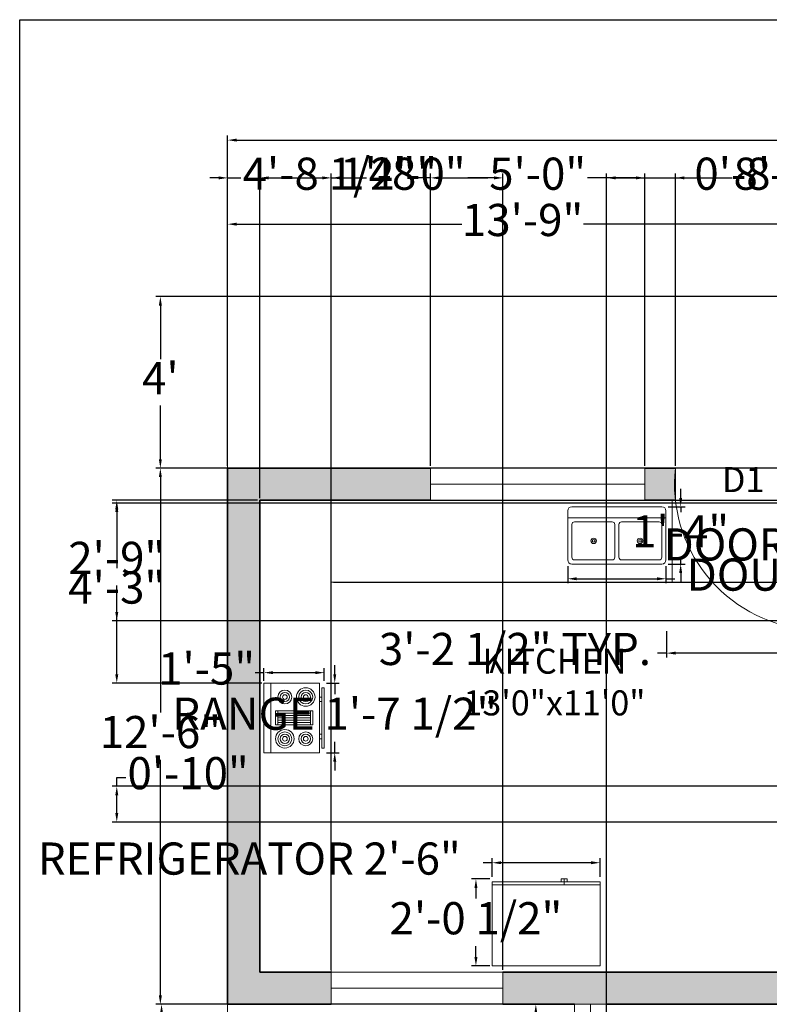
# Model space of a CAD drawing. Units: inches. Extents: x 1942 to 2601, y 2026 to 2623.
# Tile 2 of 5: x 1942 to 2151, y 2348 to 2623. Entities that reach past the tile are written whole.
import ezdxf

# ---------------------------------------------------------------- set-up
doc = ezdxf.new("R2010")
doc.units = ezdxf.units.IN
doc.linetypes.add('ACAD_ISO02W100', pattern=[15, 12, -3])
for name, color, linetype, lineweight in [('A-ANNO-DIMS', 2, 'Continuous', 18), ('A-ANNO-TEXT', 7, 'Continuous', 18), ('A-ANNO-TTLB', 7, 'Continuous', 25), ('A-AREA-IDEN', 7, 'Continuous', 25), ('A-DOOR', 4, 'Continuous', 18), ('A-EQPM', 8, 'Continuous', 18), ('A-FLOR-CASE', 8, 'Continuous', 18), ('A-FLOR-FIXT', 8, 'Continuous', 18), ('A-FLOR-OTLN', 8, 'ACAD_ISO02W100', 13), ('A-GLAZ', 2, 'Continuous', 18), ('A-WALL', 7, 'Continuous', 35), ('A-WALL-PATT', 7, 'Continuous', 13)]:
    doc.layers.add(name, color=color, linetype=linetype, lineweight=lineweight)
doc.styles.get("Standard").update_dxf_attribs({"font": 'arial.ttf'})
doc.dimstyles.new('ISO-25', dxfattribs={"dimtxt": 9, "dimasz": 2.5, "dimexe": 1.25, "dimexo": 0.625, "dimgap": 2, "dimtad": 0, "dimtih": 1, "dimtoh": 1, "dimdec": 1, "dimlunit": 4, "dimtxsty": 'Standard', "dimcen": 2.5, "dimadec": 0, "dimazin": 0, "dimtfac": 0.5, "dimtdec": 1, "dimtmove": 0, "dimatfit": 3, "dimfxl": 1, "dimarcsym": 0})

# ---------------------------------------------------------------- blocks, each defined once
blk = doc.blocks.new('Sink-double - 36 in top')
for p, q in [((-18, -4), (18, -4)), ((-0.75, -18.5), (-0.75, -6.5)), ((0.75, -6.5), (0.75, -18.5))]:
    blk.add_line(p, q)
for points in [[(-16.5, 0), (16.5, 0)], [(-18, -19.5), (-18, -1.5)], [(18, -1.5), (18, -19.5)], [(-16.5, -18.5), (-16.5, -6.5)], [(-15.5, -5.5), (-1.75, -5.5)], [(1.75, -5.5), (15.5, -5.5)], [(16.5, -6.5), (16.5, -18.5)], [(16.5, -21), (-16.5, -21)], [(-1.75, -19.5), (-15.5, -19.5)], [(15.5, -19.5), (1.75, -19.5)]]:
    blk.add_lwpolyline(points)
for centre, radius in [((-8.5, -12.5), 1), ((-8.5, -12.5), 0.5), ((8.5, -12.5), 1), ((8.5, -12.5), 0.5)]:
    blk.add_circle(centre, radius)
for centre, radius, start, end in [((-16.5, -1.5), 1.5, 90, 180), ((16.5, -1.5), 1.5, 0, 90), ((-15.5, -6.5), 1, 90, 180), ((-1.75, -6.5), 1, 0, 90), ((1.75, -6.5), 1, 90, 180), ((15.5, -6.5), 1, 0, 90), ((-16.5, -19.5), 1.5, 180, 270), ((-15.5, -18.5), 1, 180, 270), ((-1.75, -18.5), 1, 270, 0), ((1.75, -18.5), 1, 180, 270), ((15.5, -18.5), 1, 270, 0), ((16.5, -19.5), 1.5, 270, 0)]:
    blk.add_arc(centre, radius, start, end)
blk = doc.blocks.new('Refrigerator-2 door - 36 in top')
for p, q in [((0, -26.999999), (36, -26.999999)), ((11, -27.999999), (11, -28.999999)), ((11, -28.999999), (13, -28.999999)), ((12, -26.999999), (12, -28.999999)), ((13, -28.999999), (13, -27.999999))]:
    blk.add_line(p, q)
blk.add_lwpolyline([(0, -27.999999), (0, 0), (36, 0), (36, -27.999999)], close=True)
blk = doc.blocks.new('Range-Oven - 30 in top')
for p, q in [((0, -3), (30, -3)), ((12, -6), (18, -6)), ((13, -20), (13, -6)), ((14, -6), (14, -20)), ((15, -20), (15, -6)), ((16, -6), (16, -20)), ((17, -20), (17, -6)), ((18, -20), (12, -20)), ((6, -24), (6, -25)), ((8, -25), (8, -24)), ((22, -25), (22, -24)), ((24, -24), (24, -25))]:
    blk.add_line(p, q)
for points in [[(0, -24), (0, 0), (30, 0), (30, -24)], [(12, -21), (12, -5), (18, -5), (18, -21)], [(2, -26), (2, -25), (28, -25), (28, -26)]]:
    blk.add_lwpolyline(points, close=True)
for centre, radius in [((6, -9), 4), ((6, -9), 3), ((6, -9), 2), ((6, -9), 1), ((24, -9), 3), ((24, -9), 2), ((24, -9), 1), ((6, -18), 3), ((6, -18), 2), ((24, -18), 4), ((24, -18), 3), ((24, -18), 2), ((6, -18), 1), ((24, -18), 1)]:
    blk.add_circle(centre, radius)
blk = doc.blocks.new('*D12')
at = {"layer": 'A-ANNO-DIMS', "color": 0, "lineweight": -2, "transparency": 16777216}
for p, q in [((1999.82, 2498.54), (1999.82, 2567.42)), ((2164.82, 2498.54), (2164.82, 2567.42)), ((2002.32, 2566.17), (2065.28, 2566.17)), ((2162.32, 2566.17), (2099.35, 2566.17))]:
    blk.add_line(p, q, dxfattribs=at)
at = {"layer": 'A-ANNO-DIMS', "color": 0, "transparency": 16777216}
for points in [[(2002.32, 2566.58), (2002.32, 2565.75), (1999.82, 2566.17)], [(2162.32, 2566.58), (2162.32, 2565.75), (2164.82, 2566.17)]]:
    blk.add_solid(points, dxfattribs=at)
at = {"layer": 'Defpoints', "color": 0, "transparency": 16777216}
for p in [(2164.82, 2566.17), (1999.82, 2497.91), (2164.82, 2497.91)]:
    blk.add_point(p, dxfattribs=at)
at = {"layer": 'A-ANNO-DIMS', "color": 0, "transparency": 16777216, "insert": (2082.32, 2566.17), "char_height": 9, "attachment_point": 5}
blk.add_mtext('13\'-9"', dxfattribs=at)
blk = doc.blocks.new('*D14')
at = {"layer": 'A-ANNO-DIMS', "color": 0, "lineweight": -2, "transparency": 16777216}
for p, q in [((1999.82, 2498.54), (1999.82, 2590.94)), ((2002.32, 2589.69), (2224.18, 2589.69)), ((2481.32, 2589.69), (2259.46, 2589.69)), ((2483.82, 2498.54), (2483.82, 2590.94))]:
    blk.add_line(p, q, dxfattribs=at)
at = {"layer": 'A-ANNO-DIMS', "color": 0, "transparency": 16777216}
for points in [[(2002.32, 2590.1), (2002.32, 2589.27), (1999.82, 2589.69)], [(2481.32, 2590.1), (2481.32, 2589.27), (2483.82, 2589.69)]]:
    blk.add_solid(points, dxfattribs=at)
at = {"layer": 'Defpoints', "color": 0, "transparency": 16777216}
for p in [(2483.82, 2589.69), (1999.82, 2497.91), (2483.82, 2497.91)]:
    blk.add_point(p, dxfattribs=at)
at = {"layer": 'A-ANNO-DIMS', "color": 0, "transparency": 16777216, "insert": (2241.82, 2589.69), "char_height": 9, "attachment_point": 5}
blk.add_mtext('40\'-4"', dxfattribs=at)
blk = doc.blocks.new('*D15')
at = {"layer": 'A-ANNO-DIMS', "color": 0, "lineweight": -2, "transparency": 16777216}
for p, q in [((1999.19, 2497.91), (1979.76, 2497.91)), ((1981.01, 2495.41), (1981.01, 2429.51)), ((1981.01, 2350.41), (1981.01, 2416.32)), ((1999.19, 2347.91), (1979.76, 2347.91))]:
    blk.add_line(p, q, dxfattribs=at)
at = {"layer": 'A-ANNO-DIMS', "color": 0, "transparency": 16777216}
for points in [[(1980.59, 2495.41), (1981.43, 2495.41), (1981.01, 2497.91)], [(1980.59, 2350.41), (1981.43, 2350.41), (1981.01, 2347.91)]]:
    blk.add_solid(points, dxfattribs=at)
at = {"layer": 'Defpoints', "color": 0, "transparency": 16777216}
for p in [(1999.82, 2497.91), (1981.01, 2347.91), (1999.82, 2347.91)]:
    blk.add_point(p, dxfattribs=at)
at = {"layer": 'A-ANNO-DIMS', "color": 0, "transparency": 16777216, "insert": (1981.01, 2422.91), "char_height": 9, "attachment_point": 5}
blk.add_mtext('12\'-6"', dxfattribs=at)
blk = doc.blocks.new('*D16')
at = {"layer": 'A-ANNO-DIMS', "color": 0, "lineweight": -2, "transparency": 16777216}
for p, q in [((2164.19, 2545.91), (1979.76, 2545.91)), ((1981.01, 2543.41), (1981.01, 2528.41)), ((1981.01, 2500.41), (1981.01, 2515.41)), ((2164.19, 2497.91), (1979.76, 2497.91))]:
    blk.add_line(p, q, dxfattribs=at)
at = {"layer": 'A-ANNO-DIMS', "color": 0, "transparency": 16777216}
for points in [[(1980.59, 2543.41), (1981.43, 2543.41), (1981.01, 2545.91)], [(1980.59, 2500.41), (1981.43, 2500.41), (1981.01, 2497.91)]]:
    blk.add_solid(points, dxfattribs=at)
at = {"layer": 'Defpoints', "color": 0, "transparency": 16777216}
for p in [(2164.82, 2545.91), (1981.01, 2497.91), (2164.82, 2497.91)]:
    blk.add_point(p, dxfattribs=at)
at = {"layer": 'A-ANNO-DIMS', "color": 0, "transparency": 16777216, "insert": (1981.01, 2521.91), "char_height": 9, "attachment_point": 5}
blk.add_mtext("4'", dxfattribs=at)
blk = doc.blocks.new('*D17')
at = {"layer": 'A-ANNO-DIMS', "color": 0, "lineweight": -2, "transparency": 16777216}
for p, q in [((2096.19, 2347.91), (1980.09, 2347.91)), ((1981.34, 2345.41), (1981.34, 2259.51)), ((1981.34, 2160.41), (1981.34, 2246.32)), ((2096.19, 2157.91), (1980.09, 2157.91))]:
    blk.add_line(p, q, dxfattribs=at)
at = {"layer": 'A-ANNO-DIMS', "color": 0, "transparency": 16777216}
for points in [[(1980.92, 2345.41), (1981.75, 2345.41), (1981.34, 2347.91)], [(1980.92, 2160.41), (1981.75, 2160.41), (1981.34, 2157.91)]]:
    blk.add_solid(points, dxfattribs=at)
at = {"layer": 'Defpoints', "color": 0, "transparency": 16777216}
for p in [(2096.82, 2347.91), (1981.34, 2157.91), (2096.82, 2157.91)]:
    blk.add_point(p, dxfattribs=at)
at = {"layer": 'A-ANNO-DIMS', "color": 0, "transparency": 16777216, "insert": (1981.34, 2252.91), "char_height": 9, "attachment_point": 5}
blk.add_mtext('15\'-10"', dxfattribs=at)
blk = doc.blocks.new('WIN-72IN')
for p, q in [((0, 0), (0, 9)), ((0, 9), (72, 9)), ((72, 0), (72, 9)), ((0, 4.5), (72, 4.5)), ((0, 0), (72, 0))]:
    blk.add_line(p, q)
blk = doc.blocks.new('DOOR-SINGLE-36IN')
for p, q in [((0, 9), (0, 45)), ((1, 9), (1, 44.88)), ((0, 0), (0, 9)), ((36, 0), (36, 9))]:
    blk.add_line(p, q)
blk.add_arc((-4.5, 4.5), 40.75, 353.6598, 83.6598)
blk = doc.blocks.new('*D29')
at = {"layer": 'A-ANNO-DIMS', "color": 0, "lineweight": -2, "transparency": 16777216}
for p, q in [((2029.78, 2440.27), (2029.78, 2442.77)), ((2027.49, 2437.77), (2031.03, 2437.77)), ((2029.78, 2437.77), (2029.78, 2434.69)), ((2029.78, 2418.31), (2029.78, 2421.39)), ((2027.49, 2418.31), (2031.03, 2418.31)), ((2029.78, 2415.81), (2029.78, 2413.31))]:
    blk.add_line(p, q, dxfattribs=at)
at = {"layer": 'A-ANNO-DIMS', "color": 0, "transparency": 16777216}
for points in [[(2029.36, 2440.27), (2030.2, 2440.27), (2029.78, 2437.77)], [(2029.36, 2415.81), (2030.2, 2415.81), (2029.78, 2418.31)]]:
    blk.add_solid(points, dxfattribs=at)
at = {"layer": 'Defpoints', "color": 0, "transparency": 16777216}
for p in [(2026.86, 2437.77), (2029.78, 2437.77), (2026.86, 2418.31)]:
    blk.add_point(p, dxfattribs=at)
at = {"layer": 'A-ANNO-DIMS', "color": 0, "transparency": 16777216, "insert": (2029.78, 2428.04), "char_height": 9, "attachment_point": 5}
blk.add_mtext('RANGE 1\'-7 1/2"', dxfattribs=at)
blk = doc.blocks.new('*D30')
at = {"layer": 'A-ANNO-DIMS', "color": 0, "lineweight": -2, "transparency": 16777216}
for p, q in [((2009.99, 2440.69), (2007.49, 2440.69)), ((2009.99, 2438.4), (2009.99, 2441.94)), ((2024.36, 2440.69), (2012.49, 2440.69)), ((2026.86, 2438.4), (2026.86, 2441.94))]:
    blk.add_line(p, q, dxfattribs=at)
at = {"layer": 'A-ANNO-DIMS', "color": 0, "transparency": 16777216}
for points in [[(2012.49, 2441.11), (2012.49, 2440.28), (2009.99, 2440.69)], [(2024.36, 2441.11), (2024.36, 2440.28), (2026.86, 2440.69)]]:
    blk.add_solid(points, dxfattribs=at)
at = {"layer": 'Defpoints', "color": 0, "transparency": 16777216}
for p in [(2009.99, 2440.69), (2009.99, 2437.77), (2026.86, 2437.77)]:
    blk.add_point(p, dxfattribs=at)
at = {"layer": 'A-ANNO-DIMS', "color": 0, "transparency": 16777216, "insert": (1993.95, 2440.69), "char_height": 9, "attachment_point": 5}
blk.add_mtext('1\'-5"', dxfattribs=at)
blk = doc.blocks.new('*D31')
at = {"layer": 'A-ANNO-DIMS', "color": 0, "lineweight": -2, "transparency": 16777216}
for p, q in [((2096.19, 2347.91), (2084.77, 2347.91)), ((2086.02, 2345.41), (2086.02, 2318.57)), ((2086.02, 2278.41), (2086.02, 2305.26)), ((2096.19, 2275.91), (2084.77, 2275.91))]:
    blk.add_line(p, q, dxfattribs=at)
at = {"layer": 'A-ANNO-DIMS', "color": 0, "transparency": 16777216}
for points in [[(2085.6, 2345.41), (2086.44, 2345.41), (2086.02, 2347.91)], [(2085.6, 2278.41), (2086.44, 2278.41), (2086.02, 2275.91)]]:
    blk.add_solid(points, dxfattribs=at)
at = {"layer": 'Defpoints', "color": 0, "transparency": 16777216}
for p in [(2096.82, 2347.91), (2086.02, 2275.91), (2096.82, 2275.91)]:
    blk.add_point(p, dxfattribs=at)
at = {"layer": 'A-ANNO-DIMS', "color": 0, "transparency": 16777216, "insert": (2086.02, 2311.91), "char_height": 9, "attachment_point": 5}
blk.add_mtext('WINDOW 6\'-0" TYP.', dxfattribs=at)
blk = doc.blocks.new('*D35')
at = {"layer": 'A-ANNO-DIMS', "color": 0, "lineweight": -2, "transparency": 16777216}
for p, q in [((2161.7, 2497.91), (2169.07, 2497.91)), ((2167.82, 2495.41), (2167.82, 2482.07)), ((2167.82, 2455.41), (2167.82, 2468.75)), ((2161.7, 2452.91), (2169.07, 2452.91))]:
    blk.add_line(p, q, dxfattribs=at)
at = {"layer": 'A-ANNO-DIMS', "color": 0, "transparency": 16777216}
for points in [[(2167.41, 2495.41), (2168.24, 2495.41), (2167.82, 2497.91)], [(2167.41, 2455.41), (2168.24, 2455.41), (2167.82, 2452.91)]]:
    blk.add_solid(points, dxfattribs=at)
at = {"layer": 'Defpoints', "color": 0, "transparency": 16777216}
for p in [(2161.07, 2497.91), (2161.07, 2452.91), (2167.82, 2452.91)]:
    blk.add_point(p, dxfattribs=at)
at = {"layer": 'A-ANNO-DIMS', "color": 0, "transparency": 16777216, "insert": (2167.82, 2475.41), "char_height": 9, "attachment_point": 5}
blk.add_mtext('DOOR 3\'-9" TYP.', dxfattribs=at)
blk = doc.blocks.new('*D36')
at = {"layer": 'A-ANNO-DIMS', "color": 0, "lineweight": -2, "transparency": 16777216}
for p, q in [((2122.59, 2452.29), (2122.59, 2444.91)), ((2161.07, 2452.29), (2161.07, 2444.91)), ((2122.59, 2446.16), (2120.09, 2446.16)), ((2158.57, 2446.16), (2125.09, 2446.16))]:
    blk.add_line(p, q, dxfattribs=at)
at = {"layer": 'A-ANNO-DIMS', "color": 0, "transparency": 16777216}
for points in [[(2125.09, 2446.58), (2125.09, 2445.75), (2122.59, 2446.16)], [(2158.57, 2446.58), (2158.57, 2445.75), (2161.07, 2446.16)]]:
    blk.add_solid(points, dxfattribs=at)
at = {"layer": 'Defpoints', "color": 0, "transparency": 16777216}
for p in [(2122.59, 2452.91), (2161.07, 2452.91), (2122.59, 2446.16)]:
    blk.add_point(p, dxfattribs=at)
at = {"layer": 'A-ANNO-DIMS', "color": 0, "transparency": 16777216, "insert": (2080.18, 2446.16), "char_height": 9, "attachment_point": 5}
blk.add_mtext('3\'-2 1/2" TYP.', dxfattribs=at)
blk = doc.blocks.new('*D49')
at = {"layer": 'A-ANNO-DIMS', "color": 0, "lineweight": -2, "transparency": 16777216}
for p, q in [((2094.95, 2470.45), (2094.95, 2465.71)), ((2122.41, 2470.45), (2122.41, 2465.71)), ((2097.45, 2466.96), (2119.91, 2466.96)), ((2122.41, 2466.96), (2124.91, 2466.96))]:
    blk.add_line(p, q, dxfattribs=at)
at = {"layer": 'A-ANNO-DIMS', "color": 0, "transparency": 16777216}
for points in [[(2097.45, 2467.38), (2097.45, 2466.54), (2094.95, 2466.96)], [(2119.91, 2467.38), (2119.91, 2466.54), (2122.41, 2466.96)]]:
    blk.add_solid(points, dxfattribs=at)
at = {"layer": 'Defpoints', "color": 0, "transparency": 16777216}
for p in [(2094.95, 2471.08), (2122.41, 2471.08), (2122.41, 2466.96)]:
    blk.add_point(p, dxfattribs=at)
at = {"layer": 'A-ANNO-DIMS', "color": 0, "transparency": 16777216, "insert": (2193.15, 2466.96), "char_height": 9, "attachment_point": 5}
blk.add_mtext('DOUBLE SINK 2\'-3 1/2"', dxfattribs=at)
blk = doc.blocks.new('*D50')
at = {"layer": 'A-ANNO-DIMS', "color": 0, "lineweight": -2, "transparency": 16777216}
for p, q in [((2126.53, 2489.6), (2126.53, 2492.1)), ((2123.03, 2487.1), (2127.78, 2487.1)), ((2126.53, 2487.1), (2126.53, 2485.61)), ((2123.03, 2471.08), (2127.78, 2471.08)), ((2126.53, 2471.08), (2126.53, 2472.57)), ((2126.53, 2468.58), (2126.53, 2466.08))]:
    blk.add_line(p, q, dxfattribs=at)
at = {"layer": 'A-ANNO-DIMS', "color": 0, "transparency": 16777216}
for points in [[(2126.11, 2489.6), (2126.94, 2489.6), (2126.53, 2487.1)], [(2126.11, 2468.58), (2126.94, 2468.58), (2126.53, 2471.08)]]:
    blk.add_solid(points, dxfattribs=at)
at = {"layer": 'Defpoints', "color": 0, "transparency": 16777216}
for p in [(2122.41, 2487.1), (2126.53, 2487.1), (2122.41, 2471.08)]:
    blk.add_point(p, dxfattribs=at)
at = {"layer": 'A-ANNO-DIMS', "color": 0, "transparency": 16777216, "insert": (2126.53, 2479.09), "char_height": 9, "attachment_point": 5}
blk.add_mtext('1\'-4"', dxfattribs=at)
blk = doc.blocks.new('*D51')
at = {"layer": 'A-ANNO-DIMS', "color": 0, "lineweight": -2, "transparency": 16777216}
for p, q in [((2073.8, 2383.62), (2073.8, 2388.77)), ((2103.99, 2383.62), (2103.99, 2388.77)), ((2073.8, 2387.52), (2071.3, 2387.52)), ((2101.49, 2387.52), (2076.3, 2387.52))]:
    blk.add_line(p, q, dxfattribs=at)
at = {"layer": 'A-ANNO-DIMS', "color": 0, "transparency": 16777216}
for points in [[(2076.3, 2387.94), (2076.3, 2387.11), (2073.8, 2387.52)], [(2101.49, 2387.94), (2101.49, 2387.11), (2103.99, 2387.52)]]:
    blk.add_solid(points, dxfattribs=at)
at = {"layer": 'Defpoints', "color": 0, "transparency": 16777216}
for p in [(2073.8, 2387.52), (2073.8, 2382.99), (2103.99, 2382.99)]:
    blk.add_point(p, dxfattribs=at)
at = {"layer": 'A-ANNO-DIMS', "color": 0, "transparency": 16777216, "insert": (2005.88, 2387.52), "char_height": 9, "attachment_point": 5}
blk.add_mtext('REFRIGERATOR 2\'-6"', dxfattribs=at)
blk = doc.blocks.new('*D52')
at = {"layer": 'A-ANNO-DIMS', "color": 0, "lineweight": -2, "transparency": 16777216}
for p, q in [((2073.17, 2382.99), (2068.02, 2382.99)), ((2069.27, 2380.49), (2069.27, 2377.49)), ((2069.27, 2361.18), (2069.27, 2364.18)), ((2073.17, 2358.68), (2068.02, 2358.68))]:
    blk.add_line(p, q, dxfattribs=at)
at = {"layer": 'A-ANNO-DIMS', "color": 0, "transparency": 16777216}
for points in [[(2068.85, 2380.49), (2069.69, 2380.49), (2069.27, 2382.99)], [(2068.85, 2361.18), (2069.69, 2361.18), (2069.27, 2358.68)]]:
    blk.add_solid(points, dxfattribs=at)
at = {"layer": 'Defpoints', "color": 0, "transparency": 16777216}
for p in [(2073.8, 2382.99), (2069.27, 2358.68), (2073.8, 2358.68)]:
    blk.add_point(p, dxfattribs=at)
at = {"layer": 'A-ANNO-DIMS', "color": 0, "transparency": 16777216, "insert": (2069.27, 2370.83), "char_height": 9, "attachment_point": 5}
blk.add_mtext('2\'-0 1/2"', dxfattribs=at)
blk = doc.blocks.new('*D53')
at = {"layer": 'A-ANNO-DIMS', "color": 0, "lineweight": -2, "transparency": 16777216}
for p, q in [((1997.32, 2579.12), (1994.82, 2579.12)), ((1999.82, 2498.54), (1999.82, 2580.37)), ((1999.82, 2579.12), (2003.55, 2579.12)), ((2056.54, 2579.12), (2052.81, 2579.12)), ((2056.54, 2498.54), (2056.54, 2580.37)), ((2059.04, 2579.12), (2061.54, 2579.12))]:
    blk.add_line(p, q, dxfattribs=at)
at = {"layer": 'A-ANNO-DIMS', "color": 0, "transparency": 16777216}
for points in [[(1997.32, 2579.54), (1997.32, 2578.7), (1999.82, 2579.12)], [(2059.04, 2579.54), (2059.04, 2578.7), (2056.54, 2579.12)]]:
    blk.add_solid(points, dxfattribs=at)
at = {"layer": 'Defpoints', "color": 0, "transparency": 16777216}
for p in [(2056.54, 2579.12), (1999.82, 2497.91), (2056.54, 2497.91)]:
    blk.add_point(p, dxfattribs=at)
at = {"layer": 'A-ANNO-DIMS', "color": 0, "transparency": 16777216, "insert": (2028.18, 2579.12), "char_height": 9, "attachment_point": 5}
blk.add_mtext('4\'-8 1/2"', dxfattribs=at)
blk = doc.blocks.new('*D54')
at = {"layer": 'A-ANNO-DIMS', "color": 0, "lineweight": -2, "transparency": 16777216}
for p, q in [((2056.54, 2498.54), (2056.54, 2580.37)), ((2059.04, 2579.12), (2072.58, 2579.12)), ((2114.04, 2579.12), (2100.5, 2579.12)), ((2116.54, 2498.54), (2116.54, 2580.37))]:
    blk.add_line(p, q, dxfattribs=at)
at = {"layer": 'A-ANNO-DIMS', "color": 0, "transparency": 16777216}
for points in [[(2059.04, 2579.54), (2059.04, 2578.7), (2056.54, 2579.12)], [(2114.04, 2579.54), (2114.04, 2578.7), (2116.54, 2579.12)]]:
    blk.add_solid(points, dxfattribs=at)
at = {"layer": 'Defpoints', "color": 0, "transparency": 16777216}
for p in [(2116.54, 2579.12), (2056.54, 2497.91), (2116.54, 2497.91)]:
    blk.add_point(p, dxfattribs=at)
at = {"layer": 'A-ANNO-DIMS', "color": 0, "transparency": 16777216, "insert": (2086.54, 2579.12), "char_height": 9, "attachment_point": 5}
blk.add_mtext('5\'-0"', dxfattribs=at)
blk = doc.blocks.new('*D55')
at = {"layer": 'A-ANNO-DIMS', "color": 0, "lineweight": -2, "transparency": 16777216}
for p, q in [((2114.04, 2579.12), (2111.54, 2579.12)), ((2116.54, 2498.54), (2116.54, 2580.37)), ((2116.54, 2579.12), (2125.07, 2579.12)), ((2125.07, 2498.54), (2125.07, 2580.37)), ((2127.57, 2579.12), (2130.07, 2579.12))]:
    blk.add_line(p, q, dxfattribs=at)
at = {"layer": 'A-ANNO-DIMS', "color": 0, "transparency": 16777216}
for points in [[(2114.04, 2579.54), (2114.04, 2578.7), (2116.54, 2579.12)], [(2127.57, 2579.54), (2127.57, 2578.7), (2125.07, 2579.12)]]:
    blk.add_solid(points, dxfattribs=at)
at = {"layer": 'Defpoints', "color": 0, "transparency": 16777216}
for p in [(2125.07, 2579.12), (2116.54, 2497.91), (2125.07, 2497.91)]:
    blk.add_point(p, dxfattribs=at)
at = {"layer": 'A-ANNO-DIMS', "color": 0, "transparency": 16777216, "insert": (2154.52, 2579.12), "char_height": 9, "attachment_point": 5}
blk.add_mtext('0\'-8 1/2"', dxfattribs=at)
blk = doc.blocks.new('*D56')
at = {"layer": 'A-ANNO-DIMS', "color": 0, "lineweight": -2, "transparency": 16777216}
for p, q in [((2028.82, 2357.54), (2028.82, 2580.37)), ((2031.32, 2579.12), (2038.68, 2579.12)), ((2074.32, 2579.12), (2066.96, 2579.12)), ((2076.82, 2357.54), (2076.82, 2580.37))]:
    blk.add_line(p, q, dxfattribs=at)
at = {"layer": 'A-ANNO-DIMS', "color": 0, "transparency": 16777216}
for points in [[(2031.32, 2579.54), (2031.32, 2578.7), (2028.82, 2579.12)], [(2074.32, 2579.54), (2074.32, 2578.7), (2076.82, 2579.12)]]:
    blk.add_solid(points, dxfattribs=at)
at = {"layer": 'Defpoints', "color": 0, "transparency": 16777216}
for p in [(2076.82, 2579.12), (2028.82, 2356.91), (2076.82, 2356.91)]:
    blk.add_point(p, dxfattribs=at)
at = {"layer": 'A-ANNO-DIMS', "color": 0, "transparency": 16777216, "insert": (2052.82, 2579.12), "char_height": 9, "attachment_point": 5}
blk.add_mtext('4\'-0"', dxfattribs=at)
blk = doc.blocks.new('*D66')
at = {"layer": 'A-ANNO-DIMS', "color": 0, "lineweight": -2, "transparency": 16777216}
for p, q in [((2105.82, 2167.54), (2105.82, 2580.37)), ((2108.32, 2579.12), (2140.9, 2579.12)), ((2201.42, 2579.12), (2168.84, 2579.12)), ((2203.92, 2167.54), (2203.92, 2580.37))]:
    blk.add_line(p, q, dxfattribs=at)
at = {"layer": 'A-ANNO-DIMS', "color": 0, "transparency": 16777216}
for points in [[(2108.32, 2579.54), (2108.32, 2578.7), (2105.82, 2579.12)], [(2201.42, 2579.54), (2201.42, 2578.7), (2203.92, 2579.12)]]:
    blk.add_solid(points, dxfattribs=at)
at = {"layer": 'Defpoints', "color": 0, "transparency": 16777216}
for p in [(2203.92, 2579.12), (2105.82, 2166.91), (2203.92, 2166.91)]:
    blk.add_point(p, dxfattribs=at)
at = {"layer": 'A-ANNO-DIMS', "color": 0, "transparency": 16777216, "insert": (2154.87, 2579.12), "char_height": 9, "attachment_point": 5}
blk.add_mtext('8\'-2"', dxfattribs=at)
blk = doc.blocks.new('*D70')
at = {"layer": 'A-ANNO-DIMS', "color": 0, "lineweight": -2, "transparency": 16777216}
for p, q in [((1968.82, 2408.91), (1968.82, 2411.41)), ((1968.82, 2411.41), (1971.32, 2411.41)), ((2173.19, 2408.91), (1967.57, 2408.91)), ((1968.82, 2401.41), (1968.82, 2406.41)), ((2173.19, 2398.91), (1967.57, 2398.91))]:
    blk.add_line(p, q, dxfattribs=at)
at = {"layer": 'A-ANNO-DIMS', "color": 0, "transparency": 16777216}
for points in [[(1968.4, 2406.41), (1969.24, 2406.41), (1968.82, 2408.91)], [(1968.4, 2401.41), (1969.24, 2401.41), (1968.82, 2398.91)]]:
    blk.add_solid(points, dxfattribs=at)
at = {"layer": 'Defpoints', "color": 0, "transparency": 16777216}
for p in [(1968.82, 2408.91), (2173.82, 2408.91), (2173.82, 2398.91)]:
    blk.add_point(p, dxfattribs=at)
at = {"layer": 'A-ANNO-DIMS', "color": 0, "transparency": 16777216, "insert": (1988.78, 2411.41), "char_height": 9, "attachment_point": 5}
blk.add_mtext('0\'-10"', dxfattribs=at)
blk = doc.blocks.new('*D73')
at = {"layer": 'A-ANNO-DIMS', "color": 0, "lineweight": -2, "transparency": 16777216}
for p, q in [((2008.82, 2489.54), (2008.82, 2580.37)), ((2011.32, 2579.12), (2026.32, 2579.12)), ((2028.82, 2466.67), (2028.82, 2580.37)), ((2028.82, 2579.12), (2031.32, 2579.12))]:
    blk.add_line(p, q, dxfattribs=at)
at = {"layer": 'A-ANNO-DIMS', "color": 0, "transparency": 16777216}
for points in [[(2011.32, 2579.54), (2011.32, 2578.7), (2008.82, 2579.12)], [(2026.32, 2579.54), (2026.32, 2578.7), (2028.82, 2579.12)]]:
    blk.add_solid(points, dxfattribs=at)
at = {"layer": 'Defpoints', "color": 0, "transparency": 16777216}
for p in [(2028.82, 2579.12), (2008.82, 2488.91), (2028.82, 2466.05)]:
    blk.add_point(p, dxfattribs=at)
at = {"layer": 'A-ANNO-DIMS', "color": 0, "transparency": 16777216, "insert": (2044.86, 2579.12), "char_height": 9, "attachment_point": 5}
blk.add_mtext('1\'-8"', dxfattribs=at)
blk = doc.blocks.new('*D74')
at = {"layer": 'A-ANNO-DIMS', "color": 0, "lineweight": -2, "transparency": 16777216}
for p, q in [((2009.44, 2488.91), (2516.07, 2488.91)), ((2514.82, 2486.41), (2514.82, 2484)), ((2514.82, 2468.55), (2514.82, 2470.96)), ((2029.44, 2466.05), (2516.07, 2466.05))]:
    blk.add_line(p, q, dxfattribs=at)
at = {"layer": 'A-ANNO-DIMS', "color": 0, "transparency": 16777216}
for points in [[(2514.4, 2486.41), (2515.24, 2486.41), (2514.82, 2488.91)], [(2514.4, 2468.55), (2515.24, 2468.55), (2514.82, 2466.05)]]:
    blk.add_solid(points, dxfattribs=at)
at = {"layer": 'Defpoints', "color": 0, "transparency": 16777216}
for p in [(2008.82, 2488.91), (2514.82, 2488.91), (2028.82, 2466.05)]:
    blk.add_point(p, dxfattribs=at)
at = {"layer": 'A-ANNO-DIMS', "color": 0, "transparency": 16777216, "insert": (2514.82, 2477.48), "char_height": 9, "attachment_point": 5}
blk.add_mtext('1\'-11"', dxfattribs=at)
blk = doc.blocks.new('*D76')
at = {"layer": 'A-ANNO-DIMS', "color": 0, "lineweight": -2, "transparency": 16777216}
for p, q in [((2295.53, 2488.12), (1967.57, 2488.12)), ((1968.82, 2485.62), (1968.82, 2478.23)), ((1968.82, 2457.66), (1968.82, 2465.04)), ((2295, 2455.16), (1967.57, 2455.16))]:
    blk.add_line(p, q, dxfattribs=at)
at = {"layer": 'A-ANNO-DIMS', "color": 0, "transparency": 16777216}
for points in [[(1968.4, 2485.62), (1969.24, 2485.62), (1968.82, 2488.12)], [(1968.4, 2457.66), (1969.24, 2457.66), (1968.82, 2455.16)]]:
    blk.add_solid(points, dxfattribs=at)
at = {"layer": 'Defpoints', "color": 0, "transparency": 16777216}
for p in [(1968.82, 2488.12), (2296.15, 2488.12), (2295.63, 2455.16)]:
    blk.add_point(p, dxfattribs=at)
at = {"layer": 'A-ANNO-DIMS', "color": 0, "transparency": 16777216, "insert": (1968.82, 2471.64), "char_height": 9, "attachment_point": 5}
blk.add_mtext('2\'-9"', dxfattribs=at)
blk = doc.blocks.new('*D77')
at = {"layer": 'A-ANNO-DIMS', "color": 0, "lineweight": -2, "transparency": 16777216}
for p, q in [((2008.19, 2488.91), (1967.57, 2488.91)), ((1968.82, 2486.41), (1968.82, 2469.94)), ((1968.82, 2440.27), (1968.82, 2456.74)), ((2009.37, 2437.77), (1967.57, 2437.77))]:
    blk.add_line(p, q, dxfattribs=at)
at = {"layer": 'A-ANNO-DIMS', "color": 0, "transparency": 16777216}
for points in [[(1968.4, 2486.41), (1969.24, 2486.41), (1968.82, 2488.91)], [(1968.4, 2440.27), (1969.24, 2440.27), (1968.82, 2437.77)]]:
    blk.add_solid(points, dxfattribs=at)
at = {"layer": 'Defpoints', "color": 0, "transparency": 16777216}
for p in [(1968.82, 2488.91), (2008.82, 2488.91), (2009.99, 2437.77)]:
    blk.add_point(p, dxfattribs=at)
at = {"layer": 'A-ANNO-DIMS', "color": 0, "transparency": 16777216, "insert": (1968.82, 2463.34), "char_height": 9, "attachment_point": 5}
blk.add_mtext('4\'-3"', dxfattribs=at)

msp = doc.modelspace()

# ---------------------------------------------------------------- hatches: boundary and pattern name
at = {"layer": 'A-WALL-PATT'}
h = msp.add_hatch(color=256, dxfattribs=at)
h.dxf.hatch_style = 1
h.paths.add_polyline_path([(2056.54, 2497.91), (1999.82, 2497.91), (1999.82, 2347.91), (2008.82, 2347.91), (2028.82, 2347.91), (2028.82, 2356.91), (2008.82, 2356.91), (2008.82, 2488.91), (2056.54, 2488.91)])
h.paths.add_polyline_path([(2173.82, 2356.91), (2164.82, 2356.91), (2076.82, 2356.91), (2076.82, 2347.91), (2096.82, 2347.91), (2105.82, 2347.91), (2164.82, 2347.91), (2173.82, 2347.91)])
h.paths.add_polyline_path([(2173.82, 2488.91), (2173.82, 2497.91), (2173.82, 2536.91), (2179.57, 2536.91), (2179.57, 2545.91), (2173.82, 2545.91), (2164.82, 2545.91), (2164.82, 2497.91), (2161.07, 2497.91), (2161.07, 2488.91), (2164.82, 2488.91), (2164.82, 2392.91), (2173.82, 2392.91)])
h.paths.add_polyline_path([(2125.07, 2497.91), (2116.54, 2497.91), (2116.54, 2488.91), (2125.07, 2488.91, -0.055385)])
h.paths.add_polyline_path([(2266.32, 2545.91), (2257.32, 2545.91), (2251.57, 2545.91), (2251.57, 2536.91), (2257.32, 2536.91), (2257.32, 2497.91), (2257.32, 2488.91), (2257.32, 2347.91), (2318.82, 2347.91), (2342.82, 2347.91), (2342.82, 2356.91), (2318.82, 2356.91), (2318.82, 2386.91), (2314.32, 2386.91), (2314.32, 2356.91), (2266.32, 2356.91), (2266.32, 2410.91), (2289.34, 2410.91, -0.055385), (2289.34, 2416.91), (2266.32, 2416.91), (2266.32, 2488.91), (2278.32, 2488.91), (2278.32, 2497.91), (2266.32, 2497.91)])
h.paths.add_polyline_path([(2360.82, 2497.91), (2314.32, 2497.91), (2314.32, 2488.91), (2314.32, 2416.91), (2314.32, 2410.91), (2318.82, 2410.91), (2318.82, 2488.91), (2360.82, 2488.91)])
h.paths.add_polyline_path([(2483.82, 2497.91), (2432.82, 2497.91), (2432.82, 2488.91), (2474.82, 2488.91), (2474.82, 2458.91), (2483.82, 2458.91)])
h.paths.add_polyline_path([(2483.82, 2386.91), (2474.82, 2386.91), (2474.82, 2356.91), (2378.82, 2356.91, -0.055385), (2378.82, 2347.91), (2386.82, 2347.91), (2386.82, 2299.91), (2386.82, 2293.91), (2394.45, 2293.91), (2394.45, 2299.91), (2392.82, 2299.91), (2392.82, 2347.91), (2474.82, 2347.91), (2474.82, 2341.91), (2483.82, 2341.91)])
h.paths.add_polyline_path([(2483.82, 2305.91), (2474.82, 2305.91), (2474.82, 2299.91), (2418.45, 2299.91, -0.055385), (2418.45, 2293.91), (2420.82, 2293.91), (2420.82, 2285.08, -0.055385), (2426.82, 2285.08), (2426.82, 2293.91), (2474.82, 2293.91), (2474.82, 2288.91), (2483.82, 2288.91)])

# ---------------------------------------------------------------- linework, layer by layer
at = {"layer": 'A-ANNO-TTLB'}
msp.add_lwpolyline([(1941.67, 2623.37), (2601.3, 2623.37), (2601.3, 2026.31), (1941.67, 2026.31)], close=True, dxfattribs=at)
at = {"layer": 'A-FLOR-CASE'}
for p, q in [((2124.17, 2466.05), (2124.17, 2488.91)), ((2028.82, 2356.91), (2028.82, 2466.05)), ((2028.82, 2466.05), (2124.17, 2466.05))]:
    msp.add_line(p, q, dxfattribs=at)
at = {"layer": 'A-FLOR-OTLN'}
for p, q in [((2164.82, 2545.91), (1999.82, 2545.91)), ((1999.82, 2497.91), (1999.82, 2545.91)), ((1999.82, 2347.91), (1999.82, 2073.91))]:
    msp.add_line(p, q, dxfattribs=at)
at = {"layer": 'A-GLAZ'}
for p, q in [((2056.54, 2497.91), (2056.54, 2488.91)), ((2056.54, 2497.91), (2116.54, 2497.91)), ((2116.54, 2497.91), (2116.54, 2488.91)), ((2056.54, 2493.41), (2116.54, 2493.41)), ((2056.54, 2488.91), (2116.54, 2488.91)), ((2028.82, 2347.91), (2028.82, 2356.91)), ((2028.82, 2356.91), (2076.82, 2356.91)), ((2076.82, 2347.91), (2076.82, 2356.91)), ((2028.82, 2352.41), (2076.82, 2352.41)), ((2028.82, 2347.91), (2076.82, 2347.91))]:
    msp.add_line(p, q, dxfattribs=at)
at = {"layer": 'A-WALL'}
for p, q in [((1999.82, 2497.91), (2056.54, 2497.91)), ((1999.82, 2347.91), (1999.82, 2497.91)), ((2116.54, 2497.91), (2125.07, 2497.91)), ((2008.82, 2356.91), (2008.82, 2488.91)), ((2008.82, 2488.91), (2056.54, 2488.91)), ((2116.54, 2488.91), (2125.07, 2488.91)), ((2008.82, 2356.91), (2028.82, 2356.91)), ((2076.82, 2356.91), (2164.82, 2356.91)), ((2008.82, 2347.91), (1999.82, 2347.91)), ((2008.82, 2347.91), (2028.82, 2347.91)), ((2076.82, 2347.91), (2096.82, 2347.91)), ((2105.82, 2347.91), (2164.82, 2347.91))]:
    msp.add_line(p, q, dxfattribs=at)

# ---------------------------------------------------------------- block references
at = {"layer": 'A-DOOR', "rotation": 180}
msp.add_blockref('DOOR-SINGLE-36IN', (2161.07, 2497.91), dxfattribs=at)
at = {"layer": 'A-EQPM'}
for name, p, xscale, yscale, zscale, rotation in [('Range-Oven - 30 in top', (2009.99, 2418.31), 0.6488642466990004, 0.6488642466990004, 0.6488642466990004, 90), ('Refrigerator-2 door - 36 in top', (2103.99, 2358.68), 0.8385807165928312, 0.8385807165928312, 0.8385807165928312, 180)]:
    msp.add_blockref(name, p, dxfattribs=dict(at, xscale=xscale, yscale=yscale, zscale=zscale, rotation=rotation))
at = {"layer": 'A-FLOR-FIXT', "xscale": 0.7627323757076447, "yscale": 0.7627323757076447, "zscale": 0.7627323757076447}
msp.add_blockref('Sink-double - 36 in top', (2108.68, 2487.1), dxfattribs=at)
at = {"layer": 'A-GLAZ', "rotation": 269.9999999999981}
msp.add_blockref('WIN-72IN', (2096.82, 2347.91), dxfattribs=at)

# ---------------------------------------------------------------- texts
at = {"layer": 'A-ANNO-TEXT', "insert": (2135.5, 2498.2), "char_height": 7, "attachment_point": 1}
msp.add_mtext_dynamic_manual_height_columns('\\pxqc;D1', width=17.0257, gutter_width=12.5, heights=[0], dxfattribs=at)
at = {"layer": 'A-AREA-IDEN', "insert": (2040.17, 2447.41), "char_height": 7, "attachment_point": 1}
msp.add_mtext_dynamic_manual_height_columns('\\pxqc;{\\fArial|b1|i0|c0|p34;KITCHEN\\P13\'0"x11\'0"}', width=102.0991, gutter_width=12.5, heights=[0], dxfattribs=at)

# ---------------------------------------------------------------- dimensions: what is measured, and where the dimension line sits
at = {"layer": 'A-ANNO-DIMS'}
for base, p1, p2, override, picture, middle in [((2483.82, 2589.69), (1999.82, 2497.91), (2483.82, 2497.91), {"dimclrd": 0, "dimclre": 0, "dimclrt": 0}, '*D14', (2241.82, 2589.69)), ((2056.54, 2579.12), (1999.82, 2497.91), (2056.54, 2497.91), {"dimdec": 1, "dimlfac": 1, "dimrnd": 0, "dimzin": 1, "dimdsep": 46, "dimlunit": 4, "dimfrac": 2}, '*D53', (2028.18, 2579.12)), ((2125.07, 2579.12), (2116.54, 2497.91), (2125.07, 2497.91), {"dimdec": 1, "dimlfac": 1, "dimrnd": 0, "dimzin": 1, "dimdsep": 46, "dimlunit": 4, "dimfrac": 2}, '*D55', (2154.52, 2579.12)), ((2028.82, 2579.12), (2008.82, 2488.91), (2028.82, 2466.05), {"dimdec": 1, "dimlfac": 1, "dimrnd": 0, "dimzin": 1, "dimdsep": 46, "dimlunit": 4, "dimfrac": 2}, '*D73', (2044.86, 2579.12)), ((2076.82, 2579.12), (2028.82, 2356.91), (2076.82, 2356.91), {"dimdec": 1, "dimlfac": 1, "dimrnd": 0, "dimzin": 1, "dimdsep": 46, "dimlunit": 4, "dimfrac": 2}, '*D56', (2052.82, 2579.12)), ((2116.54, 2579.12), (2056.54, 2497.91), (2116.54, 2497.91), {"dimdec": 1, "dimlfac": 1, "dimrnd": 0, "dimzin": 1, "dimdsep": 46, "dimlunit": 4, "dimfrac": 2}, '*D54', (2086.54, 2579.12)), ((2203.92, 2579.12), (2105.82, 2166.91), (2203.92, 2166.91), {"dimdec": 1, "dimlfac": 1, "dimrnd": 0, "dimzin": 1, "dimdsep": 46, "dimlunit": 4, "dimfrac": 2}, '*D66', (2154.87, 2579.12)), ((2164.82, 2566.17), (1999.82, 2497.91), (2164.82, 2497.91), {"dimclrd": 0, "dimclre": 0, "dimclrt": 0}, '*D12', (2082.32, 2566.17))]:
    dim = msp.add_linear_dim(base=base, p1=p1, p2=p2, dimstyle='ISO-25', override=override, dxfattribs=at)
    dim.commit()
    dim.dimension.update_dxf_attribs({"geometry": picture, "text_midpoint": middle})
for base, p1, p2, angle, override, picture, middle in [((1981.01, 2497.91), (2164.82, 2545.91), (2164.82, 2497.91), 90, {"dimclrd": 0, "dimclre": 0, "dimclrt": 0}, '*D16', (1981.01, 2521.91)), ((2126.53, 2487.1), (2122.41, 2471.08), (2122.41, 2487.1), 90, {"dimdec": 1, "dimlfac": 1, "dimrnd": 0, "dimzin": 1, "dimdsep": 46, "dimlunit": 4, "dimfrac": 2}, '*D50', (2126.53, 2479.09)), ((1968.82, 2488.91), (2009.99, 2437.77), (2008.82, 2488.91), 90, {"dimdec": 1, "dimlfac": 1, "dimrnd": 0, "dimzin": 1, "dimdsep": 46, "dimlunit": 4, "dimfrac": 2}, '*D77', (1968.82, 2463.34)), ((1968.82, 2488.12), (2295.63, 2455.16), (2296.15, 2488.12), 90, {"dimdec": 1, "dimlfac": 1, "dimrnd": 0, "dimzin": 1, "dimdsep": 46, "dimlunit": 4, "dimfrac": 2}, '*D76', (1968.82, 2471.64)), ((2514.82, 2488.91), (2028.82, 2466.05), (2008.82, 2488.91), 90, {"dimdec": 1, "dimlfac": 1, "dimrnd": 0, "dimzin": 1, "dimdsep": 46, "dimlunit": 4, "dimfrac": 2}, '*D74', (2514.82, 2477.48)), ((2009.99, 2440.69), (2026.86, 2437.77), (2009.99, 2437.77), 180, {"dimdec": 1, "dimlfac": 1, "dimrnd": 0, "dimzin": 1, "dimdsep": 46, "dimlunit": 4, "dimfrac": 2}, '*D30', (1993.95, 2440.69)), ((1968.82, 2408.91), (2173.82, 2398.91), (2173.82, 2408.91), 90, {"dimdec": 1, "dimlfac": 1, "dimrnd": 0, "dimzin": 1, "dimdsep": 46, "dimlunit": 4, "dimfrac": 2}, '*D70', (1988.78, 2411.41)), ((2069.27, 2358.68), (2073.8, 2382.99), (2073.8, 2358.68), 270, {"dimdec": 1, "dimlfac": 1, "dimrnd": 0, "dimzin": 1, "dimdsep": 46, "dimlunit": 4, "dimfrac": 2}, '*D52', (2069.27, 2370.83)), ((1981.34, 2157.91), (2096.82, 2347.91), (2096.82, 2157.91), 90, {"dimclrd": 0, "dimclre": 0, "dimclrt": 0}, '*D17', (1981.34, 2252.91))]:
    dim = msp.add_linear_dim(base=base, p1=p1, p2=p2, angle=angle, dimstyle='ISO-25', override=override, dxfattribs=at)
    dim.commit()
    dim.dimension.update_dxf_attribs({"geometry": picture, "text_midpoint": middle})
dim = msp.add_aligned_dim(p1=(1999.82, 2497.91), p2=(1999.82, 2347.91), distance=-18.81, dimstyle='ISO-25', override={"dimclrd": 0, "dimclre": 0, "dimclrt": 0}, dxfattribs=at)
dim.commit()
dim.dimension.update_dxf_attribs({"geometry": '*D15', "text_midpoint": (1981.01, 2422.91)})
for base, p1, p2, angle, text, picture, middle in [((2167.82, 2452.91), (2161.07, 2497.91), (2161.07, 2452.91), 270, 'DOOR <> TYP.', '*D35', (2167.82, 2475.41)), ((2122.59, 2446.16), (2161.07, 2452.91), (2122.59, 2452.91), 180, '<> TYP.', '*D36', (2080.18, 2446.16)), ((2029.78, 2437.77), (2026.86, 2418.31), (2026.86, 2437.77), 90, 'RANGE <>', '*D29', (2029.78, 2428.04)), ((2073.8, 2387.52), (2103.99, 2382.99), (2073.8, 2382.99), 180, 'REFRIGERATOR <>', '*D51', (2005.88, 2387.52)), ((2086.02, 2275.91), (2096.82, 2347.91), (2096.82, 2275.91), 270, 'WINDOW <> TYP.', '*D31', (2086.02, 2311.91))]:
    dim = msp.add_linear_dim(base=base, p1=p1, p2=p2, angle=angle, text=text, dimstyle='ISO-25', override={"dimdec": 1, "dimlfac": 1, "dimrnd": 0, "dimzin": 1, "dimdsep": 46, "dimlunit": 4, "dimfrac": 2}, dxfattribs=at)
    dim.commit()
    dim.dimension.update_dxf_attribs({"geometry": picture, "text_midpoint": middle})
dim = msp.add_linear_dim(base=(2122.41, 2466.96), p1=(2094.95, 2471.08), p2=(2122.41, 2471.08), text='DOUBLE SINK <>', dimstyle='ISO-25', override={"dimdec": 1, "dimlfac": 1, "dimrnd": 0, "dimzin": 1, "dimdsep": 46, "dimlunit": 4, "dimfrac": 2}, dxfattribs=at)
dim.commit()
dim.dimension.update_dxf_attribs({"geometry": '*D49', "text_midpoint": (2193.15, 2466.96)})

doc.saveas('drawing.dxf')
